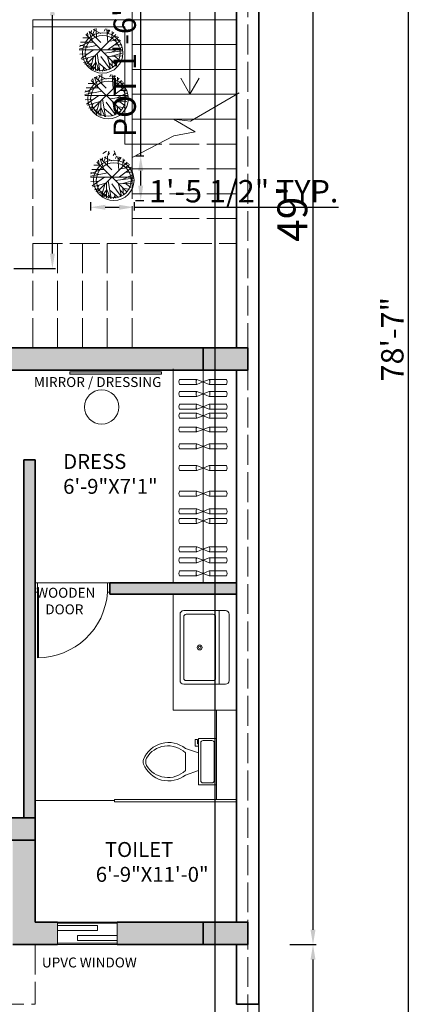
# Model space of a CAD drawing. Units: millimetres. Extents: x 595116 to 630915, y 909473 to 920225.
# Tile 121 of 134: x 629746 to 629904, y 919346 to 919742. Entities that reach past the tile are written whole.
import ezdxf

# ---------------------------------------------------------------- set-up
doc = ezdxf.new("R2010")
doc.units = ezdxf.units.MM
doc.linetypes.add('ACAD_ISO02W100', pattern=[15, 12, -3])
for name, color, linetype, lineweight in [('A-ANNO-SYMB', 7, 'Continuous', 18), ('A-AREA-IDEN', 7, 'Continuous', 20), ('A-FLOR-FIXT', 9, 'Continuous', 18), ('A-FLOR-OVHD', 253, 'ACAD_ISO02W100', 13), ('A-FLOR-STRS-HIDN', 142, 'ACAD_ISO02W100', 13), ('A-FURN', 32, 'Continuous', 18), ('A-WALL', 1, 'Continuous', 35), ('A-WALL-PATT', 8, 'Continuous', 13), ('C-PROP', 7, 'Continuous', 25), ('C-PROP-REF', 240, 'ACAD_ISO02W100', 13), ('Column', 6, 'Continuous', 35), ('Dimension', 3, 'Continuous', 18), ('Doors', 31, 'Continuous', 20), ('L-PLNT', 85, 'Continuous', 13), ('STAIR CASE', 142, 'Continuous', 20), ('Text', 7, 'Continuous', 18), ('Windows', 33, 'Continuous', 18)]:
    doc.layers.add(name, color=color, linetype=linetype, lineweight=lineweight)
doc.styles.get("Standard").update_dxf_attribs({"font": 'arial.ttf'})
doc.dimstyles.new('ISO-25', dxfattribs={"dimtxt": 9, "dimasz": 6, "dimexe": 1.25, "dimexo": 0.625, "dimtad": 1, "dimlunit": 4, "dimtxsty": 'Standard', "dimcen": 2.5, "dimadec": 0, "dimazin": 0, "dimtfac": 1, "dimtmove": 0, "dimatfit": 3, "dimfxl": 1, "dimarcsym": 0})

# ---------------------------------------------------------------- blocks, each defined once
blk = doc.blocks.new('DS')
blk.add_lwpolyline([(630069.78, 919993.92), (630069.78, 919965.68), (630069.37, 919965.68), (630069.37, 919993.91)])
for points in [[(630041.6, 919963.81), (630041.6, 919967.56), (630040.69, 919967.56), (630040.69, 919963.81)], [(630069.78, 919963.81), (630070.69, 919963.81), (630070.69, 919967.56), (630069.78, 919967.56)]]:
    blk.add_lwpolyline(points, close=True)
blk.add_arc((630069.78, 919965.69), 28.24, 89.99, 176.196)
blk = doc.blocks.new('Toilet - top')
for p, q in [((9.5, -6), (9.5, -2)), ((-10, -8.5), (-8, -8.5)), ((-10, -9.5), (-10, -8.5)), ((-8, -8.5), (-8, -8)), ((-7, -8), (-7, -9.5)), ((-4, -8), (-6, -14)), ((4, -8), (6, -14)), ((-7, -9.5), (-10, -9.5)), ((4, -14), (-4, -14))]:
    blk.add_line(p, q)
blk.add_lwpolyline([(10.5, -8), (10.5, 0), (-10.5, 0), (-10.5, -8)], close=True)
for points in [[(-9.5, -2), (-9.5, -6)], [(8.5, -1), (-8.5, -1)], [(-8.5, -7), (8.5, -7)]]:
    blk.add_lwpolyline(points)
for centre, radius, start, end in [((-8.62, -1.88), 0.884, 81.8699, 188.1301), ((8.62, -1.88), 0.884, 351.8699, 98.1301), ((-8.62, -6.12), 0.884, 171.8699, 278.1301), ((8.62, -6.12), 0.884, 261.8699, 8.1301), ((3.52, -21.58), 12.17, 141.4691, 247.9714), ((4.2, -21.82), 11.33, 136.3677, 238.9468), ((-3.52, -21.58), 12.17, 292.0284, 38.5307), ((-4.2, -21.82), 11.33, 301.053, 43.6321), ((0, -27.88), 4, 245.7318, 294.2682), ((0, -29), 4, 254.8605, 285.1395)]:
    blk.add_arc(centre, radius, start, end)
blk = doc.blocks.new('Sink-single - 30 in top')
blk.add_line((-15, -3.999996), (15, -3.999996))
for points in [[(-13.5, 0), (13.5, 0)], [(-15, -18.499996), (-15, -1.5)], [(15, -1.5), (15, -18.499996)], [(-13.5, -17.499996), (-13.5, -6.499996)], [(-12.5, -5.499996), (12.5, -5.499996)], [(13.5, -6.499996), (13.5, -17.499996)], [(13.5, -19.999996), (-13.5, -19.999996)], [(12.5, -18.499996), (-12.5, -18.499996)]]:
    blk.add_lwpolyline(points)
for radius in [1, 0.5]:
    blk.add_circle((0, -11.999996), radius)
for centre, radius, start, end in [((-13.5, -1.5), 1.5, 90, 180), ((13.5, -1.5), 1.5, 0, 90), ((-12.5, -6.499996), 1, 90, 180), ((12.5, -6.499996), 1, 0, 90), ((-13.5, -18.499996), 1.5, 180, 270), ((-12.5, -17.499996), 1, 180, 270), ((12.5, -17.499996), 1, 270, 0), ((13.5, -18.499996), 1.5, 270, 0)]:
    blk.add_arc(centre, radius, start, end)
blk = doc.blocks.new('*D122')
at = {"layer": 'Defpoints', "color": 0, "transparency": 16777216}
for p in [(629862.34, 919957.93), (629854.28, 919369.93), (629864.28, 919369.93)]:
    blk.add_point(p, dxfattribs=at)
at = {"layer": 'Dimension', "color": 0, "lineweight": -2, "transparency": 16777216}
for p, q in [((629862.97, 919957.93), (629865.53, 919957.93)), ((629864.28, 919951.93), (629864.28, 919375.93)), ((629854.9, 919369.93), (629865.53, 919369.93))]:
    blk.add_line(p, q, dxfattribs=at)
at = {"layer": 'Dimension', "color": 0, "transparency": 16777216}
for points in [[(629863.28, 919951.93), (629865.28, 919951.93), (629864.28, 919957.93)], [(629863.28, 919375.93), (629865.28, 919375.93), (629864.28, 919369.93)]]:
    blk.add_solid(points, dxfattribs=at)
at = {"layer": 'Dimension', "color": 0, "transparency": 16777216, "insert": (629857.53, 919663.93), "char_height": 12, "attachment_point": 5, "rotation": 90}
blk.add_mtext("49'", dxfattribs=at)
blk = doc.blocks.new('*D123')
at = {"layer": 'Defpoints', "color": 0, "transparency": 16777216}
for p in [(629864.28, 919369.93), (629864.28, 919141.93), (629864.28, 919141.93)]:
    blk.add_point(p, dxfattribs=at)
at = {"layer": 'Dimension', "color": 0, "lineweight": -2, "transparency": 16777216}
for p, q in [((629864.91, 919369.93), (629865.53, 919369.93)), ((629864.28, 919363.93), (629864.28, 919147.93)), ((629864.91, 919141.93), (629865.53, 919141.93))]:
    blk.add_line(p, q, dxfattribs=at)
at = {"layer": 'Dimension', "color": 0, "transparency": 16777216}
for points in [[(629863.28, 919363.93), (629865.28, 919363.93), (629864.28, 919369.93)], [(629863.28, 919147.93), (629865.28, 919147.93), (629864.28, 919141.93)]]:
    blk.add_solid(points, dxfattribs=at)
at = {"layer": 'Dimension', "color": 0, "transparency": 16777216, "insert": (629857.53, 919255.93), "char_height": 12, "attachment_point": 5, "rotation": 90}
blk.add_mtext("19'", dxfattribs=at)
blk = doc.blocks.new('*D124')
at = {"layer": 'Defpoints', "color": 0, "transparency": 16777216}
for p in [(629865.75, 920084.93), (629865.75, 919141.93), (629902.57, 919141.93)]:
    blk.add_point(p, dxfattribs=at)
at = {"layer": 'Dimension', "color": 0, "lineweight": -2, "transparency": 16777216}
for p, q in [((629866.37, 920084.93), (629903.82, 920084.93)), ((629902.57, 920078.93), (629902.57, 919147.93)), ((629866.37, 919141.93), (629903.82, 919141.93))]:
    blk.add_line(p, q, dxfattribs=at)
at = {"layer": 'Dimension', "color": 0, "transparency": 16777216}
for points in [[(629901.57, 920078.93), (629903.57, 920078.93), (629902.57, 920084.93)], [(629901.57, 919147.93), (629903.57, 919147.93), (629902.57, 919141.93)]]:
    blk.add_solid(points, dxfattribs=at)
at = {"layer": 'Dimension', "color": 0, "transparency": 16777216, "insert": (629897.35, 919613.43), "char_height": 9, "attachment_point": 5, "rotation": 90}
blk.add_mtext('78\'-7"', dxfattribs=at)
blk = doc.blocks.new('WARDROBE-HANGER')
for p, q in [((9.73, 1), (9.73, 1)), ((9.73, 1), (12.27, 0)), ((9.73, 1), (9.73, 1)), ((12.27, 2), (19.15, 2)), ((0.32, 0), (7.19, 0)), ((12.27, 0), (19.15, 0))]:
    blk.add_line(p, q)
for points in [[(7.19, 2), (0.32, 2, 0.315389), (0.32, 0)], [(9.73, 1), (7.19, 2, 0.225748), (7.19, 0), (9.73, 1), (12.27, 2)]]:
    blk.add_lwpolyline(points, format="xyb")
for centre, radius, start, end in [((10.17, 1), 2.33, 334.5576, 25.4424), ((17.71, 1), 1.74, 324.9906, 35.0094)]:
    blk.add_arc(centre, radius, start, end)
blk = doc.blocks.new('POTTED-PLANT-SMALL')
for p, q in [((2.87, 15.88), (3.4, 15.68)), ((3.32, 16.24), (3.58, 14.57)), ((3.96, 16.73), (5.31, 12.84)), ((4.16, 16.82), (8.64, 12.35)), ((4.85, 16.17), (4.88, 17.21)), ((5.49, 15.52), (6.28, 17.77)), ((5.61, 17.51), (8.67, 15.94)), ((6.89, 14.08), (6.86, 17.93)), ((10.09, 16.89), (10.53, 17.9)), ((11.52, 12.26), (11.03, 17.77)), ((11.14, 16.82), (12.03, 17.41)), ((11.24, 15.75), (12.36, 17.28)), ((13.25, 16.79), (13.05, 13.85)), ((13.17, 15.58), (13.86, 16.4)), ((4.01, 12.42), (0.12, 10.79)), ((0.57, 12.45), (5.66, 12.45)), ((1.47, 14.18), (3.93, 14.18)), ((14.75, 15.51), (2.6, 3.36)), ((14.75, 3.36), (2.6, 15.51)), ((16.53, 13.1), (11.7, 9.48)), ((12.05, 12.81), (16.38, 13.4)), ((13.91, 13.07), (15.74, 14.51)), ((14.04, 14.8), (15.41, 14.87)), ((0, 9.44), (17.35, 9.44)), ((0.04, 9.84), (6.94, 11.18)), ((0.19, 11.28), (3.48, 10.53)), ((0.78, 5.86), (5.74, 9.45)), ((7.22, 7.98), (8.31, 0.8)), ((10.02, 8.11), (17.3, 9.03)), ((12.49, 6.77), (17.19, 8.01)), ((12.92, 8.47), (17.27, 10.46)), ((14.24, 11.37), (17.09, 11.41)), ((0.22, 7.65), (3.4, 7.75)), ((0.98, 5.47), (6.25, 7.03)), ((3.98, 4.75), (1.72, 4.29)), ((3.48, 6.19), (2.31, 3.58)), ((5.1, 3.97), (3.07, 2.83)), ((5.79, 6.51), (4.54, 1.81)), ((6.56, 4.2), (4.67, 1.78)), ((6.53, 7.26), (6.56, 1.1)), ((6.56, 4.78), (8.11, 0.84)), ((7.78, 4.2), (11.26, 1.19)), ((8.67, 6.68), (12.41, 1.65)), ((11.37, 6.74), (12.54, 1.72)), ((11.39, 6.74), (16.97, 6.94)), ((11.98, 4.16), (13.78, 2.43)), ((13.07, 5.08), (13.35, 2.21)), ((13.22, 4.91), (15.85, 4.62)), ((14.19, 6.81), (16.25, 5.24)), ((4.88, 3.09), (3.65, 2.4)), ((6.56, 2.6), (5.05, 1.59)), ((5.56, 2.86), (5.79, 1.32)), ((7.45, 2.56), (7.01, 0.97)), ((7.75, 1.81), (7.32, 0.93)), ((9.89, 1.75), (9.23, 0.84)), ((9.53, 2.7), (10.2, 0.97)), ((12.26, 2.96), (12, 1.49))]:
    blk.add_line(p, q)
for radius in [8.14, 7.03]:
    blk.add_circle((9.43, 8.14), radius)
blk = doc.blocks.new('COLUMN-RECT-18X9')
h = blk.add_hatch(color=256)
h.dxf.hatch_style = 1
h.paths.add_polyline_path([(18, 9), (0, 9), (0, 0), (18, 0)])
blk.add_lwpolyline([(0, 9), (18, 9), (18, 0), (0, 0)], close=True)
blk = doc.blocks.new('*D180')
at = {"layer": 'Defpoints', "color": 0, "transparency": 16777216}
for p in [(629743.29, 919749.69), (629759.47, 919749.69), (629743.29, 919641.85)]:
    blk.add_point(p, dxfattribs=at)
at = {"layer": 'Dimension', "color": 0, "lineweight": -2, "transparency": 16777216}
for p, q in [((629759.47, 919749.69), (629759.47, 919886.8)), ((629743.92, 919749.69), (629760.72, 919749.69)), ((629759.47, 919647.85), (629759.47, 919743.69)), ((629743.92, 919641.85), (629760.72, 919641.85))]:
    blk.add_line(p, q, dxfattribs=at)
at = {"layer": 'Dimension', "color": 0, "transparency": 16777216}
for points in [[(629758.47, 919743.69), (629760.47, 919743.69), (629759.47, 919749.69)], [(629758.47, 919647.85), (629760.47, 919647.85), (629759.47, 919641.85)]]:
    blk.add_solid(points, dxfattribs=at)
at = {"layer": 'Dimension', "color": 0, "transparency": 16777216, "insert": (629754.19, 919821.24), "char_height": 9, "attachment_point": 5, "rotation": 90}
blk.add_mtext('DINING SET 9\'-0" TYP.', dxfattribs=at)
blk = doc.blocks.new('*D208')
at = {"layer": 'Defpoints', "color": 0, "transparency": 16777216}
for p in [(629792.3, 919687.12), (629794.99, 919687.12), (629792.3, 919669.18)]:
    blk.add_point(p, dxfattribs=at)
at = {"layer": 'Dimension', "color": 0, "lineweight": -2, "transparency": 16777216}
for p, q in [((629794.99, 919687.12), (629794.99, 919778.12)), ((629792.93, 919687.12), (629796.24, 919687.12)), ((629794.99, 919675.18), (629794.99, 919681.12)), ((629792.93, 919669.18), (629796.24, 919669.18))]:
    blk.add_line(p, q, dxfattribs=at)
at = {"layer": 'Dimension', "color": 0, "transparency": 16777216}
for points in [[(629793.99, 919681.12), (629795.99, 919681.12), (629794.99, 919687.12)], [(629793.99, 919675.18), (629795.99, 919675.18), (629794.99, 919669.18)]]:
    blk.add_solid(points, dxfattribs=at)
at = {"layer": 'Dimension', "color": 0, "transparency": 16777216, "insert": (629789.71, 919735.62), "char_height": 9, "attachment_point": 5, "rotation": 90}
blk.add_mtext('POT 1\'-6" TYP.', dxfattribs=at)
blk = doc.blocks.new('*D209')
at = {"layer": 'Defpoints', "color": 0, "transparency": 16777216}
for p in [(629774.73, 919669.18), (629792.3, 919669.18), (629792.3, 919666.49)]:
    blk.add_point(p, dxfattribs=at)
at = {"layer": 'Dimension', "color": 0, "lineweight": -2, "transparency": 16777216}
for p, q in [((629774.73, 919668.56), (629774.73, 919665.24)), ((629780.73, 919666.49), (629786.3, 919666.49)), ((629792.3, 919668.56), (629792.3, 919665.24)), ((629792.3, 919666.49), (629874.54, 919666.49))]:
    blk.add_line(p, q, dxfattribs=at)
at = {"layer": 'Dimension', "color": 0, "transparency": 16777216}
for points in [[(629780.73, 919667.49), (629780.73, 919665.49), (629774.73, 919666.49)], [(629786.3, 919667.49), (629786.3, 919665.49), (629792.3, 919666.49)]]:
    blk.add_solid(points, dxfattribs=at)
at = {"layer": 'Dimension', "color": 0, "transparency": 16777216, "insert": (629836.42, 919671.77), "char_height": 9, "attachment_point": 5}
blk.add_mtext('1\'-5 1/2" TYP.', dxfattribs=at)
blk = doc.blocks.new('*D220')
at = {"layer": 'Defpoints', "color": 0, "transparency": 16777216}
for p in [(629824.95, 920160.76), (629511.27, 919302.01), (629824.95, 919302.01)]:
    blk.add_point(p, dxfattribs=at)
at = {"layer": 'Dimension', "color": 0, "lineweight": -2, "transparency": 16777216}
for p, q in [((629511.27, 919302.63), (629511.27, 920162.01)), ((629824.95, 919302.63), (629824.95, 920162.01)), ((629517.27, 920160.76), (629818.95, 920160.76))]:
    blk.add_line(p, q, dxfattribs=at)
at = {"layer": 'Dimension', "color": 0, "transparency": 16777216}
for points in [[(629517.27, 920161.76), (629517.27, 920159.76), (629511.27, 920160.76)], [(629818.95, 920161.76), (629818.95, 920159.76), (629824.95, 920160.76)]]:
    blk.add_solid(points, dxfattribs=at)
at = {"layer": 'Dimension', "color": 0, "transparency": 16777216, "insert": (629668.11, 920166.03), "char_height": 9, "attachment_point": 5}
blk.add_mtext('26\'-1 1/2"', dxfattribs=at)

msp = doc.modelspace()

# ---------------------------------------------------------------- hatches: boundary and pattern name
at = {"layer": 'A-FURN'}
h = msp.add_hatch(color=256, dxfattribs=at)
h.dxf.hatch_style = 1
h.paths.add_polyline_path([(629803.312, 919600.264), (629766.465, 919600.264), (629766.465, 919599.365), (629803.312, 919599.365)])
at = {"layer": 'A-WALL-PATT'}
h = msp.add_hatch(color=256, dxfattribs=at)
h.dxf.hatch_style = 1
h.paths.add_polyline_path([(629820.041, 919609.928), (629643.041, 919609.928), (629643.041, 919600.928), (629820.041, 919600.928)])
h = msp.add_hatch(color=256, dxfattribs=at)
h.dxf.hatch_style = 1
h.paths.add_polyline_path([(629752.541, 919564.928), (629748.041, 919564.928), (629748.041, 919420.928), (629752.541, 919420.928)])
h = msp.add_hatch(color=256, dxfattribs=at)
h.dxf.hatch_style = 1
h.paths.add_polyline_path([(629833.541, 919515.428), (629782.541, 919515.428), (629782.541, 919510.928), (629833.541, 919510.928)])
h = msp.add_hatch(color=256, dxfattribs=at)
h.dxf.hatch_style = 1
h.paths.add_polyline_path([(629752.541, 919411.928), (629743.541, 919411.928), (629743.541, 919369.928), (629761.541, 919369.928), (629761.541, 919378.928), (629752.541, 919378.928)])
h = msp.add_hatch(color=256, dxfattribs=at)
h.dxf.hatch_style = 1
h.paths.add_polyline_path([(629820.041, 919378.928), (629785.541, 919378.928), (629785.541, 919369.928), (629820.041, 919369.928)])

# ---------------------------------------------------------------- linework, layer by layer
at = {"layer": 'A-ANNO-SYMB'}
for p, q in [((629814.804, 919762.246), (629814.804, 919711.928)), ((629814.804, 919711.928), (629811.137, 919718.393)), ((629814.804, 919711.928), (629818.472, 919718.393))]:
    msp.add_line(p, q, dxfattribs=at)
at = {"layer": 'A-FLOR-FIXT'}
for p, q in [((629808.041, 919510.928), (629808.041, 919464.269)), ((629808.041, 919464.269), (629833.541, 919464.269)), ((629825.432, 919464.269), (629825.432, 919428.297)), ((629784.41, 919427.855), (629752.541, 919427.855)), ((629833.541, 919428.297), (629784.41, 919428.297)), ((629784.41, 919428.297), (629784.41, 919427.413)), ((629833.541, 919427.413), (629784.41, 919427.413))]:
    msp.add_line(p, q, dxfattribs=at)
at = {"layer": 'A-FLOR-OVHD'}
for p in [(629752.541, 919369.928), (629586.041, 919345.928)]:
    msp.add_line(p, (629752.541, 919345.928), dxfattribs=at)
at = {"layer": 'A-FLOR-STRS-HIDN'}
for p, q in [((629751.541, 919741.928), (629751.541, 919651.928)), ((629791.541, 919691.928), (629833.541, 919691.928)), ((629791.541, 919681.928), (629791.541, 919691.928)), ((629791.541, 919681.928), (629833.541, 919681.928)), ((629791.541, 919681.928), (629791.541, 919609.928)), ((629791.541, 919671.928), (629833.541, 919671.928)), ((629791.541, 919661.928), (629833.541, 919661.928)), ((629751.541, 919651.928), (629833.541, 919651.928)), ((629751.541, 919651.928), (629751.541, 919609.928)), ((629761.541, 919651.928), (629761.541, 919609.928)), ((629771.541, 919651.928), (629771.541, 919609.928)), ((629781.541, 919651.928), (629781.541, 919609.928))]:
    msp.add_line(p, q, dxfattribs=at)
at = {"layer": 'A-FURN'}
for p, q in [((629808.041, 919515.428), (629808.041, 919601.519)), ((629820.041, 919600.928), (629820.041, 919515.428))]:
    msp.add_line(p, q, dxfattribs=at)
msp.add_lwpolyline([(629766.465, 919600.264), (629803.312, 919600.264), (629803.312, 919599.365), (629766.465, 919599.365)], close=True, dxfattribs=at)
msp.add_circle((629779.273, 919586.157), 6.897, dxfattribs=at)
at = {"layer": 'A-WALL'}
for p, q in [((629833.541, 919783.928), (629833.541, 919609.928)), ((629643.041, 919609.928), (629838.041, 919609.928)), ((629643.041, 919600.928), (629838.041, 919600.928)), ((629833.541, 919600.928), (629833.541, 919378.928)), ((629748.041, 919564.928), (629748.041, 919420.928)), ((629748.041, 919564.928), (629752.541, 919564.928)), ((629752.541, 919564.928), (629752.541, 919378.928)), ((629782.541, 919515.428), (629833.541, 919515.428)), ((629782.541, 919515.428), (629782.541, 919510.928)), ((629782.541, 919510.928), (629833.541, 919510.928)), ((629691.041, 919420.928), (629752.541, 919420.928)), ((629752.541, 919378.928), (629761.541, 919378.928)), ((629785.541, 919378.928), (629838.041, 919378.928)), ((629743.541, 919369.928), (629761.541, 919369.928)), ((629785.541, 919369.928), (629838.041, 919369.928)), ((629833.541, 919369.928), (629833.541, 919345.928)), ((629833.541, 919345.928), (629842.541, 919345.928))]:
    msp.add_line(p, q, dxfattribs=at)
msp.add_lwpolyline([(629842.541, 919957.928), (629842.541, 919345.928)], dxfattribs=at)
at = {"layer": 'C-PROP'}
msp.add_line((629842.541, 919345.928), (629842.541, 919141.928), dxfattribs=at)
at = {"layer": 'C-PROP-REF'}
msp.add_line((629838.041, 920084.928), (629838.041, 919141.928), dxfattribs=at)
at = {"layer": 'Doors'}
msp.add_line((629753.452, 919515.428), (629781.63, 919515.428), dxfattribs=at)
at = {"layer": 'L-PLNT'}
for p, q in [((629775.77, 919718.265), (629776.025, 919716.601)), ((629776.406, 919718.755), (629777.755, 919714.872)), ((629776.61, 919718.853), (629781.089, 919714.383)), ((629777.297, 919718.2), (629777.323, 919719.244)), ((629777.933, 919717.548), (629778.722, 919719.799)), ((629778.061, 919719.538), (629781.115, 919717.972)), ((629779.333, 919716.112), (629779.308, 919719.962)), ((629782.54, 919718.918), (629782.973, 919719.929)), ((629783.965, 919714.285), (629783.482, 919719.799)), ((629783.584, 919718.853), (629784.474, 919719.44)), ((629783.685, 919717.776), (629784.805, 919719.31)), ((629785.696, 919718.82), (629785.493, 919715.883)), ((629785.62, 919717.613), (629786.307, 919718.429)), ((629776.457, 919714.448), (629772.563, 919712.816)), ((629773.021, 919714.48), (629778.112, 919714.48)), ((629773.912, 919716.21), (629776.381, 919716.21)), ((629787.192, 919717.537), (629775.049, 919705.393)), ((629787.192, 919705.393), (629775.049, 919717.537)), ((629775.312, 919717.906), (629775.846, 919717.711)), ((629788.979, 919715.133), (629784.144, 919711.511)), ((629784.5, 919714.839), (629788.827, 919715.427)), ((629786.358, 919715.1), (629788.19, 919716.536)), ((629786.485, 919716.83), (629787.86, 919716.895)), ((629772.447, 919711.465), (629789.794, 919711.465)), ((629772.487, 919711.87), (629779.384, 919713.208)), ((629772.64, 919713.306), (629775.923, 919712.555)), ((629773.225, 919707.889), (629778.188, 919711.479)), ((629779.664, 919710.01), (629780.759, 919702.832)), ((629782.464, 919710.141), (629789.743, 919711.054)), ((629784.933, 919708.803), (629789.641, 919710.043)), ((629785.365, 919710.5), (629789.717, 919712.49)), ((629786.689, 919713.404), (629789.539, 919713.436)), ((629772.665, 919709.684), (629775.846, 919709.782)), ((629773.429, 919707.498), (629778.697, 919709.064)), ((629776.432, 919706.78), (629774.167, 919706.323)), ((629775.923, 919708.216), (629774.752, 919705.605)), ((629778.239, 919708.542), (629776.992, 919703.843)), ((629779.002, 919706.225), (629777.119, 919703.811)), ((629778.977, 919709.292), (629779.002, 919703.126)), ((629779.002, 919706.813), (629780.555, 919702.864)), ((629780.224, 919706.225), (629783.711, 919703.223)), ((629781.115, 919708.705), (629784.856, 919703.68)), ((629783.813, 919708.77), (629784.984, 919703.745)), ((629783.838, 919708.77), (629789.412, 919708.966)), ((629784.424, 919706.193), (629786.231, 919704.463)), ((629785.518, 919707.106), (629785.798, 919704.235)), ((629785.671, 919706.943), (629788.292, 919706.649)), ((629786.638, 919708.836), (629788.699, 919707.269)), ((629777.552, 919705.997), (629775.516, 919704.855)), ((629777.323, 919705.116), (629776.101, 919704.431)), ((629778.01, 919704.888), (629778.239, 919703.354)), ((629784.704, 919704.985), (629784.449, 919703.517)), ((629781.284, 919689.098), (629779.782, 919688.087)), ((629782.175, 919689.066), (629781.742, 919687.467)), ((629782.48, 919688.315), (629782.048, 919687.434)), ((629784.618, 919688.25), (629783.956, 919687.336)), ((629784.262, 919689.196), (629784.924, 919687.467))]:
    msp.add_line(p, q, dxfattribs=at)
for radius in [8.14, 7.029]:
    msp.add_circle((629781.882, 919710.169), radius, dxfattribs=at)
at = {"layer": 'STAIR CASE'}
for p, q in [((629791.541, 919783.928), (629791.541, 919741.928)), ((629751.541, 919741.928), (629791.541, 919741.928)), ((629791.541, 919741.928), (629791.541, 919731.928)), ((629791.541, 919741.928), (629833.541, 919741.928)), ((629751.541, 919739.028), (629788.641, 919739.028)), ((629788.641, 919739.028), (629788.641, 919691.928)), ((629791.541, 919731.928), (629833.541, 919731.928)), ((629791.541, 919731.928), (629791.541, 919691.928)), ((629791.541, 919721.928), (629833.541, 919721.928)), ((629791.541, 919711.928), (629833.541, 919711.928)), ((629791.541, 919701.928), (629833.541, 919701.928)), ((629788.641, 919691.928), (629791.541, 919691.928))]:
    msp.add_line(p, q, dxfattribs=at)
msp.add_lwpolyline([(629791.541, 919686.489), (629808.265, 919695.169), (629816.892, 919696.774), (629808.238, 919701.928), (629814.959, 919701.125), (629834.617, 919712.564)], dxfattribs=at)
at = {"layer": 'Windows'}
for p, q in [((629761.541, 919378.928), (629761.541, 919369.928)), ((629761.541, 919378.928), (629785.541, 919378.928)), ((629761.541, 919377.598), (629777.541, 919377.598)), ((629785.541, 919378.928), (629785.541, 919369.928)), ((629761.541, 919369.928), (629785.541, 919369.928))]:
    msp.add_line(p, q, dxfattribs=at)
msp.add_lwpolyline([(629761.541, 919378.563), (629785.541, 919378.563), (629785.541, 919370.578), (629761.541, 919370.578)], close=True, dxfattribs=at)
for points in [[(629761.541, 919375.598), (629777.541, 919375.598), (629777.541, 919377.598)], [(629785.541, 919371.598), (629769.541, 919371.598), (629769.541, 919373.598), (629785.541, 919373.598)]]:
    msp.add_lwpolyline(points, dxfattribs=at)

# ---------------------------------------------------------------- block references
at = {"layer": 'A-FLOR-FIXT', "rotation": 270}
for name, p, xscale, yscale, zscale in [('Sink-single - 30 in top', (629830.538, 919489.459), 0.9872623020467125, 0.9872623020467125, 0.9872623020467125), ('Toilet - top', (629825.432, 919443.502), 0.8924547258250047, 0.8924547258250047, 0.8924547258250047)]:
    msp.add_blockref(name, p, dxfattribs=dict(at, xscale=xscale, yscale=yscale, zscale=zscale))
at = {"layer": 'A-FURN'}
for p in [(629810.307, 919595.256), (629810.314, 919590.427), (629810.314, 919585.249), (629810.314, 919581.668), (629810.314, 919576.108), (629810.314, 919569.305), (629810.314, 919560.611), (629810.314, 919550.313), (629810.314, 919543.148), (629810.314, 919539.355), (629810.307, 919527.928), (629810.314, 919523.527), (629810.314, 919518.233)]:
    msp.add_blockref('WARDROBE-HANGER', p, dxfattribs=at)
at = {"layer": 'Column'}
for p in [(629820.041, 919600.928), (629734.541, 919411.928), (629820.041, 919369.928)]:
    msp.add_blockref('COLUMN-RECT-18X9', p, dxfattribs=at)
at = {"layer": 'Doors', "rotation": 180}
msp.add_blockref('DS', (1259823.235, 1839479.237), dxfattribs=at)
at = {"layer": 'L-PLNT'}
for p in [(629770.263, 919720.416), (629774.728, 919669.183)]:
    msp.add_blockref('POTTED-PLANT-SMALL', p, dxfattribs=at)

# ---------------------------------------------------------------- texts
at = {"layer": 'A-AREA-IDEN', "char_height": 6, "attachment_point": 1}
for s, width, insert in [('{    DRESS\\P6\'-9"X7\'1"}', 14.2531, (629763.788, 919567.241)), ('{      TOILET\\P    6\'-9"X11\'-0"}', 83.57324, (629769.571, 919411.193))]:
    msp.add_mtext_dynamic_manual_height_columns(s, width=width, gutter_width=12.5, heights=[0], dxfattribs=dict(at, insert=insert))
at = {"layer": 'Text', "char_height": 4, "attachment_point": 1}
for s, width, insert in [('{     MIRROR / DRESSING}', 72.55106, (629745.93, 919598.196)), ('{     WOODEN\\P        DOOR}', 61.33456, (629746.834, 919513.444)), ('{ UPVC WINDOW}', 61.33456, (629754.022, 919364.753))]:
    msp.add_mtext_dynamic_manual_height_columns(s, width=width, gutter_width=12.5, heights=[0], dxfattribs=dict(at, insert=insert))

# ---------------------------------------------------------------- dimensions: what is measured, and where the dimension line sits
at = {"layer": 'Dimension'}
dim = msp.add_linear_dim(base=(629824.951, 920160.756), p1=(629511.274, 919302.009), p2=(629824.951, 919302.009), dimstyle='ISO-25', override={"dimdec": 1, "dimlfac": 1, "dimrnd": 0, "dimzin": 1, "dimdsep": 46, "dimlunit": 4, "dimfrac": 2}, dxfattribs=at)
dim.commit()
dim.dimension.update_dxf_attribs({"geometry": '*D220', "text_midpoint": (629668.113, 920166.035)})
for base, p1, p2, override, picture, middle in [((629902.574, 919141.928), (629865.746, 920084.928), (629865.746, 919141.928), {"dimclrd": 0, "dimclre": 0, "dimclrt": 0}, '*D124', (629897.354, 919613.428)), ((629864.281, 919369.928), (629862.344, 919957.928), (629854.278, 919369.928), {"dimtxt": 12, "dimclrd": 0, "dimclre": 0, "dimclrt": 0}, '*D122', (629857.529, 919663.928)), ((629864.281, 919141.928), (629864.281, 919369.928), (629864.281, 919141.928), {"dimtxt": 12, "dimclrd": 0, "dimclre": 0, "dimclrt": 0}, '*D123', (629857.529, 919255.928))]:
    dim = msp.add_linear_dim(base=base, p1=p1, p2=p2, angle=90, dimstyle='ISO-25', override=override, dxfattribs=at)
    dim.commit()
    dim.dimension.update_dxf_attribs({"geometry": picture, "text_midpoint": middle})
for base, p1, p2, text, picture, middle in [((629759.47, 919749.69), (629743.294, 919641.853), (629743.294, 919749.69), 'DINING SET <> TYP.', '*D180', (629754.191, 919821.242)), ((629794.994, 919687.116), (629792.304, 919669.183), (629792.304, 919687.116), 'POT <> TYP.', '*D208', (629789.712, 919735.616))]:
    dim = msp.add_linear_dim(base=base, p1=p1, p2=p2, angle=90, text=text, dimstyle='ISO-25', override={"dimdec": 1, "dimlfac": 1, "dimrnd": 0, "dimzin": 1, "dimdsep": 46, "dimlunit": 4, "dimfrac": 2}, dxfattribs=at)
    dim.commit()
    dim.dimension.update_dxf_attribs({"geometry": picture, "text_midpoint": middle})
dim = msp.add_linear_dim(base=(629792.304, 919666.493), p1=(629774.728, 919669.183), p2=(629792.304, 919669.183), text='<> TYP.', dimstyle='ISO-25', override={"dimdec": 1, "dimlfac": 1, "dimrnd": 0, "dimzin": 1, "dimdsep": 46, "dimlunit": 4, "dimfrac": 2}, dxfattribs=at)
dim.commit()
dim.dimension.update_dxf_attribs({"geometry": '*D209', "text_midpoint": (629836.42, 919671.771)})

doc.saveas('drawing.dxf')
